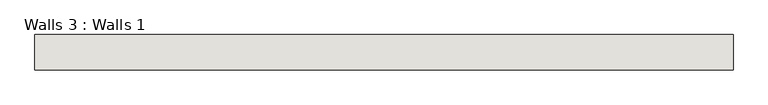
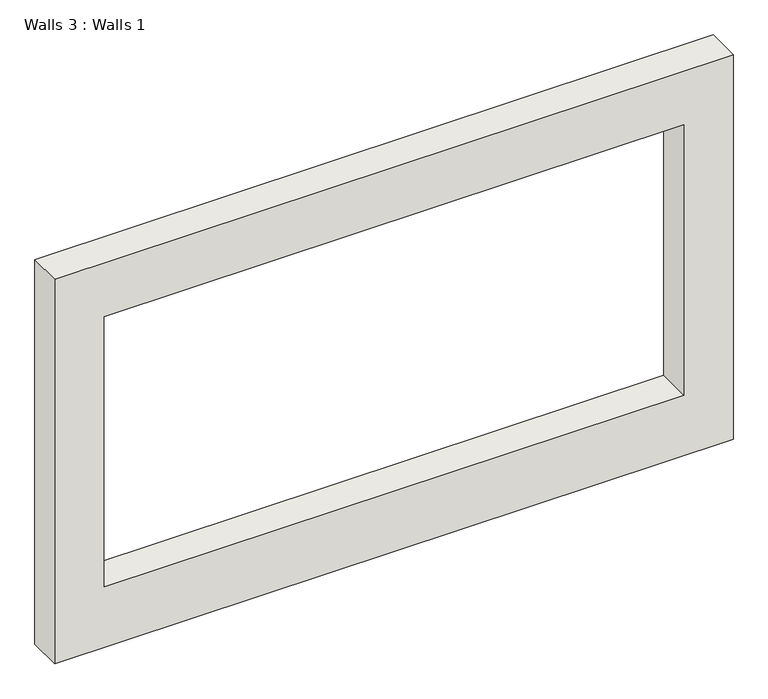
"""IFC4 building model written with IfcOpenShell, lengths in millimetres: wall geometry, Walls 3 : Walls 1."""

from ifc_helpers import new_model, si_unit, frame, origin, place, context, project, spatial, polyline, outline, extrude, source, transform, mapped, element, save


def walls_3_walls_1_396bf1f7(model_context):
    return source(origin(), model_context, "Body", "SweptSolid", [
        extrude(outline(polyline([(12254.2637952, -197.9561565), (12254.2637952, -6243.1561565), (8630.7490705, -6243.1561565), (8630.7490705, -197.9561565), (12254.2637952, -197.9561565)]), holes=[polyline([(11745.5537538, -5801.573767), (11745.5537538, -639.538546), (9201.3855951, -639.538546), (9201.3855951, -5801.573767), (11745.5537538, -5801.573767)])]), frame((0.0, 1141.3485991, 0.0), z_axis=(0.0, 1.0, 0.0), x_axis=(0.0, 0.0, 1.0)), (0.0, 0.0, 1.0), 304.8),
    ])


if __name__ == "__main__":
    model = new_model("IFC4")
    model_context = context("Model", 3, world=origin())
    ifc_project = project(units=[si_unit("LENGTHUNIT", "METRE", prefix="MILLI")], contexts=[model_context])
    site = spatial("IfcSite", under=ifc_project)
    building = spatial("IfcBuilding", under=site)
    placement = place(None, origin())
    walls_3_walls_1_shape = walls_3_walls_1_396bf1f7(model_context)
    element("IfcWall", 1, ObjectType="Walls 3 : Walls 1", at=placement, inside=building, context=model_context, shape_type="MappedRepresentation", body=[
        mapped(walls_3_walls_1_shape, transform((0.0, 0.0, 0.0), x_axis=(1.0, 0.0, 0.0), y_axis=(0.0, 1.0, 0.0), z_axis=(0.0, 0.0, 1.0))),
    ])
    save(model, "model.ifc")

# Revit data of these elements
# Element 1 (IfcWall, "Walls 3 : Walls 1")
#   Materials on its faces: "Default Wall"
# Materials
#   "Default Wall": colour RGB 128 128 128, transparency 0
